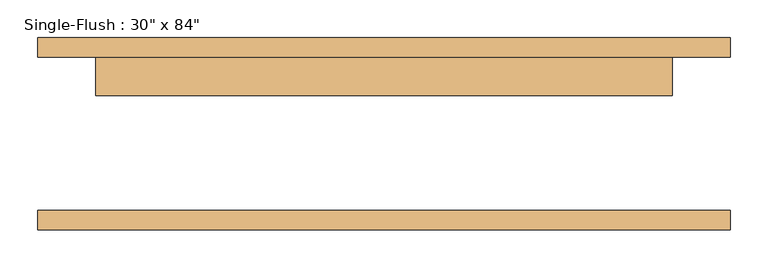
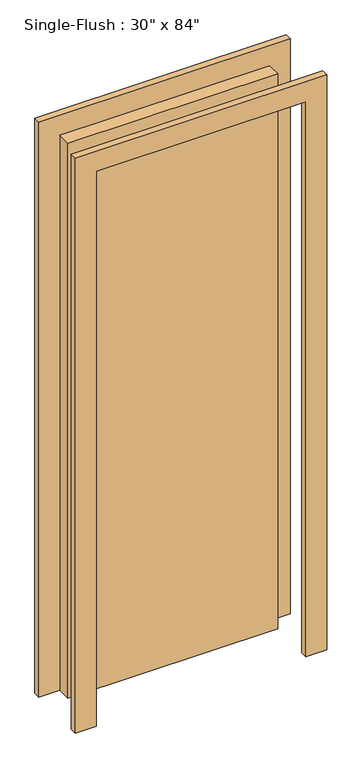
"""IFC4 building model written with IfcOpenShell, lengths in millimetres: door geometry."""

from ifc_helpers import new_model, si_unit, frame, origin, origin_with_axes, place, context, project, spatial, polyline, outline, extrude, source, transform, mapped, element, save


def door_b6acaa4e(model_context):
    return source(origin(), model_context, "Body", "SweptSolid", [
        extrude(outline(polyline([(2209.8, -457.2), (0.0, -457.2), (0.0, -381.0), (2133.6, -381.0), (2133.6, 381.0), (0.0, 381.0), (0.0, 457.2), (2209.8, 457.2), (2209.8, -457.2)])), frame((0.0, 101.6, 0.0), z_axis=(0.0, 1.0, 0.0), x_axis=(0.0, 0.0, 1.0)), (0.0, 0.0, 1.0), 25.4),
        extrude(outline(polyline([(2209.8, 457.2), (2209.8, -457.2), (0.0, -457.2), (0.0, -381.0), (2133.6, -381.0), (2133.6, 381.0), (0.0, 381.0), (0.0, 457.2), (2209.8, 457.2)])), frame((0.0, -127.0, 0.0), z_axis=(0.0, 1.0, 0.0), x_axis=(0.0, 0.0, 1.0)), (0.0, 0.0, 1.0), 25.4),
        extrude(outline(polyline([(381.0, 50.8), (-381.0, 50.8), (-381.0, 101.6), (381.0, 101.6), (381.0, 50.8)])), origin_with_axes(), (0.0, 0.0, 1.0), 2133.6),
    ])


if __name__ == "__main__":
    model = new_model("IFC4")
    model_context = context("Model", 3, world=origin())
    ifc_project = project(units=[si_unit("LENGTHUNIT", "METRE", prefix="MILLI")], contexts=[model_context])
    site = spatial("IfcSite", under=ifc_project)
    building = spatial("IfcBuilding", under=site)
    placement = place(None, origin())
    door_shape = door_b6acaa4e(model_context)
    element("IfcDoor", 1, ObjectType="Single-Flush : 30\" x 84\"", at=placement, inside=building, context=model_context, shape_type="MappedRepresentation", body=[
        mapped(door_shape, transform((0.0, 0.0, 0.0), x_axis=(1.0, 0.0, 0.0), y_axis=(0.0, 1.0, 0.0), z_axis=(0.0, 0.0, 1.0))),
    ])
    save(model, "model.ifc")

# Revit data of these elements
# Type "Single-Flush : 30\" x 84\""
#   Type Mark = "4"
#   Construction Type Id = "MDOOR"
#   Assembly Code = "C1020"
#   Analytic Construction = "Metal"
#   Thickness = 0' - 2"
#   Heat Transfer Coefficient (U) = 0.651978 BTU/(h·ft²·°F)
#   Height = 7' - 0"
#   Trim Projection Ext = 0' - 1"
#   Trim Projection Int = 0' - 1"
#   Trim Width = 0' - 3"
#   Width = 2' - 6"
#   Define Thermal Properties by = 1
#   Define Thermal Properties by = 1
#   Door Material = Door - Panel
#   Frame Material = Door - Frame
#   Visual Light Transmittance = 0
#   Solar Heat Gain Coefficient = 0
#   Function = (empty or 0)
#   Wall Closure = (empty or 0)
# Element 1 (IfcDoor, "Single-Flush : 30\" x 84\"")
#   Materials on its faces: "Door - Frame", "Door - Panel"
# Materials
#   "Door - Panel": class "Wood", colour RGB 210 159 95, transparency 0, Cost = 0
#   "Door - Frame": colour RGB 118 70 51, transparency 0, Cost = 0
